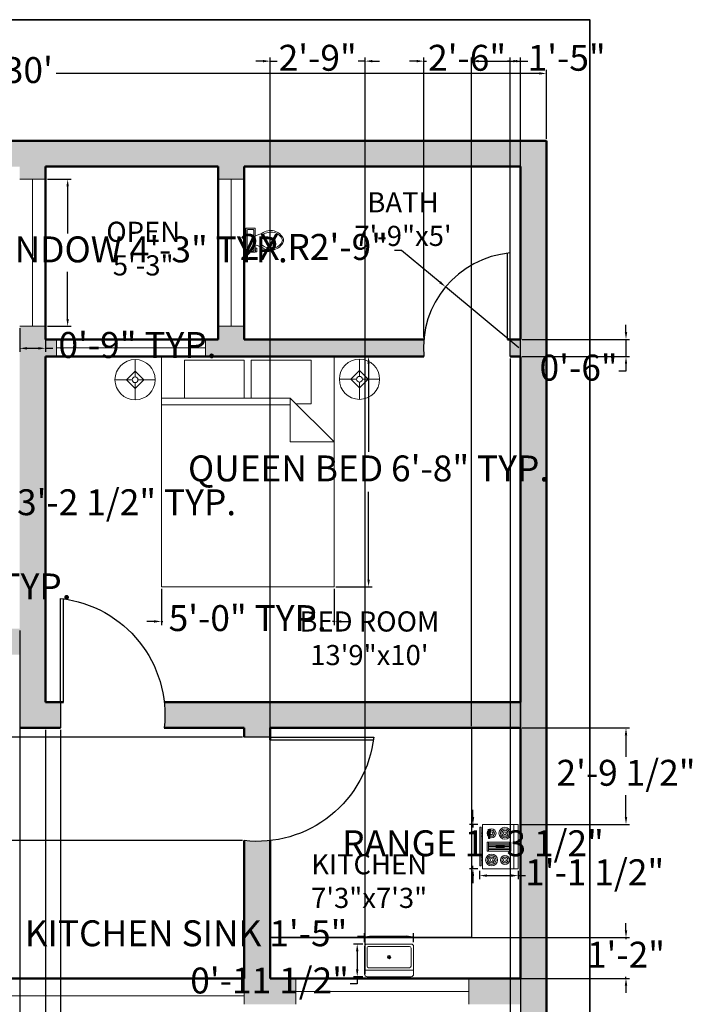
# Model space of a CAD drawing. Units: inches. Extents: x 3695 to 4182, y 4462 to 5050.
# Tile 3 of 3: x 3948 to 4182, y 4708 to 5050. Entities that reach past the tile are written whole.
import ezdxf

# ---------------------------------------------------------------- set-up
doc = ezdxf.new("R2010")
doc.units = ezdxf.units.IN
for name, color, linetype, lineweight in [('A-ANNO-DIMS', 2, 'Continuous', 18), ('A-ANNO-TTLB', 7, 'Continuous', 35), ('A-AREA-IDEN', 7, 'Continuous', 25), ('A-DOOR', 3, 'Continuous', 25), ('A-EQPM', 8, 'Continuous', 18), ('A-FLOR-CASE', 8, 'Continuous', 25), ('A-FLOR-FIXT', 9, 'Continuous', 18), ('A-FURN', 8, 'Continuous', 18), ('A-GLAZ', 4, 'Continuous', 18), ('A-WALL', 7, 'Continuous', 50)]:
    doc.layers.add(name, color=color, linetype=linetype, lineweight=lineweight)
doc.layers.add('A-WALL-PATT', color=18, linetype='Continuous', lineweight=13, true_color=0x000000)
doc.styles.get("Standard").update_dxf_attribs({"font": 'arial.ttf'})
doc.dimstyles.new('ISO-25', dxfattribs={"dimtxt": 9, "dimasz": 2.5, "dimexe": 1.25, "dimexo": 0.625, "dimgap": 2, "dimtad": 0, "dimtih": 1, "dimtoh": 1, "dimdec": 1, "dimlunit": 4, "dimtxsty": 'Standard', "dimcen": 2.5, "dimadec": 0, "dimazin": 0, "dimtfac": 0.5, "dimtdec": 1, "dimtmove": 0, "dimatfit": 3, "dimfxl": 1, "dimarcsym": 0})

# ---------------------------------------------------------------- blocks, each defined once
blk = doc.blocks.new('Bed - Queen')
for p, q in [((0, -80.00003), (0, 0)), ((0, 0), (59.99999, 0)), ((59.99999, 0), (59.99999, -80.00003)), ((7.99999, -1.2), (28.79998, -1.2)), ((7.99999, -14.4), (7.99999, -1.2)), ((28.79998, -1.2), (28.79998, -14.4)), ((31.19999, -1.2), (51.99999, -1.2)), ((31.19999, -14.4), (31.19999, -1.2)), ((51.99999, -1.2), (51.99999, -16.4)), ((0, -14.4), (44.8, -14.4)), ((44.8, -16.8), (0, -16.8)), ((59.99999, -29.6), (44.8, -14.4)), ((44.8, -14.4), (44.8, -29.6)), ((51.99999, -16.4), (46.79936, -16.4)), ((44.8, -29.6), (59.99999, -29.6)), ((59.99999, -80.00003), (0, -80.00003))]:
    blk.add_line(p, q)
blk = doc.blocks.new('Range-Oven - 30 in top')
for p, q in [((0, -3), (30, -3)), ((12, -6), (18, -6)), ((13, -20), (13, -6)), ((14, -6), (14, -20)), ((15, -20), (15, -6)), ((16, -6), (16, -20)), ((17, -20), (17, -6)), ((6, -24), (6, -25)), ((8, -25), (8, -24)), ((18, -20), (12, -20)), ((22, -25), (22, -24)), ((24, -24), (24, -25))]:
    blk.add_line(p, q)
for points in [[(0, -24), (0, 0), (30, 0), (30, -24)], [(12, -21), (12, -5), (18, -5), (18, -21)], [(2, -26), (2, -25), (28, -25), (28, -26)]]:
    blk.add_lwpolyline(points, close=True)
for centre, radius in [((6, -9), 4), ((6, -9), 3), ((24, -9), 3), ((6, -9), 2), ((6, -9), 1), ((24, -9), 2), ((24, -9), 1), ((6, -18), 3), ((6, -18), 2), ((6, -18), 1), ((24, -18), 4), ((24, -18), 3), ((24, -18), 2), ((24, -18), 1)]:
    blk.add_circle(centre, radius)
blk = doc.blocks.new('Sink-single - 30 in top')
blk.add_line((-15, -3.999996), (15, -3.999996))
for points in [[(-13.5, 0), (13.5, 0)], [(-15, -18.499996), (-15, -1.5)], [(-12.5, -5.499996), (12.5, -5.499996)], [(15, -1.5), (15, -18.499996)], [(-13.5, -17.499996), (-13.5, -6.499996)], [(13.5, -6.499996), (13.5, -17.499996)], [(13.5, -19.999996), (-13.5, -19.999996)], [(12.5, -18.499996), (-12.5, -18.499996)]]:
    blk.add_lwpolyline(points)
for radius in [1, 0.5]:
    blk.add_circle((0, -11.999996), radius)
for centre, radius, start, end in [((-13.5, -1.5), 1.5, 90, 180), ((-12.5, -6.499996), 1, 90, 180), ((12.5, -6.499996), 1, 0, 90), ((13.5, -1.5), 1.5, 0, 90), ((-12.5, -17.499996), 1, 180, 270), ((12.5, -17.499996), 1, 270, 0), ((-13.5, -18.499996), 1.5, 180, 270), ((13.5, -18.499996), 1.5, 270, 0)]:
    blk.add_arc(centre, radius, start, end)
blk = doc.blocks.new('*U7')
for p, q in [((-10, -8.5), (-8, -8.5)), ((-10, -9.5), (-10, -8.5)), ((-8, -8.5), (-8, -8)), ((-7, -8), (-7, -9.5)), ((-4, -8), (-6, -14)), ((4, -8), (6, -14)), ((9.5, -6), (9.5, -2)), ((-7, -9.5), (-10, -9.5)), ((4, -14), (-4, -14))]:
    blk.add_line(p, q)
blk.add_lwpolyline([(10.5, -8), (10.5, 0), (-10.5, 0), (-10.5, -8)], close=True)
for points in [[(-9.5, -2), (-9.5, -6)], [(8.5, -1), (-8.5, -1)], [(-8.5, -7), (8.5, -7)]]:
    blk.add_lwpolyline(points)
for centre, radius, start, end in [((-8.62, -1.88), 0.884, 81.8699, 188.1301), ((-8.62, -6.12), 0.884, 171.8699, 278.1301), ((8.62, -1.88), 0.884, 351.8699, 98.1301), ((8.62, -6.12), 0.884, 261.8699, 8.1301), ((3.52, -21.58), 12.17, 141.46911, 247.97143), ((4.2, -21.82), 11.33, 136.36773, 238.94682), ((-3.52, -21.58), 12.17, 292.02843, 38.53071), ((-4.2, -21.82), 11.33, 301.05301, 43.63209), ((0, -27.88), 4, 245.73182, 294.26817), ((0, -29), 4, 254.86053, 285.13947)]:
    blk.add_arc(centre, radius, start, end)
blk = doc.blocks.new('Lamp - Table')
for p, q in [((0, 7), (0, 1)), ((-1, 0), (-7, 0)), ((0, 3), (-3, 0)), ((-3, 0), (0, -3)), ((3, 0), (0, 3)), ((0, -3), (3, 0)), ((1, 0), (7, 0)), ((0, -1), (0, -7))]:
    blk.add_line(p, q)
for radius in [7, 1]:
    blk.add_circle((0, 0), radius)
blk = doc.blocks.new('*D11')
at = {"layer": 'A-ANNO-DIMS', "color": 0, "lineweight": -2, "transparency": 16777216}
for p, q in [((3770.96, 5008.15), (3770.96, 5032.15)), ((4130.96, 5008.15), (4130.96, 5032.15)), ((3773.46, 5030.9), (3941.33, 5030.9)), ((4128.46, 5030.9), (3960.6, 5030.9))]:
    blk.add_line(p, q, dxfattribs=at)
at = {"layer": 'A-ANNO-DIMS', "color": 0, "transparency": 16777216}
for points in [[(3773.46, 5031.31), (3773.46, 5030.48), (3770.96, 5030.9)], [(4128.46, 5031.31), (4128.46, 5030.48), (4130.96, 5030.9)]]:
    blk.add_solid(points, dxfattribs=at)
at = {"layer": 'Defpoints', "color": 0, "transparency": 16777216}
for p in [(4130.96, 5030.9), (3770.96, 5007.52), (4130.96, 5007.52)]:
    blk.add_point(p, dxfattribs=at)
at = {"layer": 'A-ANNO-DIMS', "color": 0, "transparency": 16777216, "insert": (3950.96, 5030.9), "char_height": 9, "attachment_point": 5}
blk.add_mtext("30'", dxfattribs=at)
blk = doc.blocks.new('DOOR-SINGLE-36IN')
for p, q in [((35.25, 9), (35.25, 45)), ((36.25, 9), (36.25, 45)), ((36.25, 9), (36.25, 0))]:
    blk.add_line(p, q)
blk.add_arc((40.75, 4.5), 40.75, 96.3402, 186.3402)
blk = doc.blocks.new('WIN-OPEN-COURT-51IN')
for p, q in [((9, 51.07), (0, 51.07)), ((4.5, 51.07), (4.5, 0)), ((9, 0), (0, 0))]:
    blk.add_line(p, q)
blk = doc.blocks.new('*D17')
at = {"layer": 'A-ANNO-DIMS', "color": 0, "lineweight": -2, "transparency": 16777216}
for p, q in [((3903.58, 4874.02), (3896.2, 4874.02)), ((3897.45, 4871.52), (3897.45, 4858.18)), ((3897.45, 4831.52), (3897.45, 4844.86)), ((3903.58, 4829.02), (3896.2, 4829.02))]:
    blk.add_line(p, q, dxfattribs=at)
at = {"layer": 'A-ANNO-DIMS', "color": 0, "transparency": 16777216}
for points in [[(3897.04, 4871.52), (3897.87, 4871.52), (3897.45, 4874.02)], [(3897.04, 4831.52), (3897.87, 4831.52), (3897.45, 4829.02)]]:
    blk.add_solid(points, dxfattribs=at)
at = {"layer": 'Defpoints', "color": 0, "transparency": 16777216}
for p in [(3897.45, 4874.02), (3904.2, 4874.02), (3904.2, 4829.02)]:
    blk.add_point(p, dxfattribs=at)
at = {"layer": 'A-ANNO-DIMS', "color": 0, "transparency": 16777216, "insert": (3897.45, 4851.52), "char_height": 9, "attachment_point": 5}
blk.add_mtext('SINGLE DOOR 3\'-9" TYP.', dxfattribs=at)
blk = doc.blocks.new('*D18')
at = {"layer": 'A-ANNO-DIMS', "color": 0, "lineweight": -2, "transparency": 16777216}
for p, q in [((3904.2, 4874.65), (3904.2, 4882.02)), ((3942.69, 4874.65), (3942.69, 4882.02)), ((3906.7, 4880.77), (3940.19, 4880.77)), ((3942.69, 4880.77), (3945.19, 4880.77))]:
    blk.add_line(p, q, dxfattribs=at)
at = {"layer": 'A-ANNO-DIMS', "color": 0, "transparency": 16777216}
for points in [[(3906.7, 4881.19), (3906.7, 4880.36), (3904.2, 4880.77)], [(3940.19, 4881.19), (3940.19, 4880.36), (3942.69, 4880.77)]]:
    blk.add_solid(points, dxfattribs=at)
at = {"layer": 'Defpoints', "color": 0, "transparency": 16777216}
for p in [(3942.69, 4880.77), (3904.2, 4874.02), (3942.69, 4874.02)]:
    blk.add_point(p, dxfattribs=at)
at = {"layer": 'A-ANNO-DIMS', "color": 0, "transparency": 16777216, "insert": (3985.1, 4880.77), "char_height": 9, "attachment_point": 5}
blk.add_mtext('3\'-2 1/2" TYP.', dxfattribs=at)
blk = doc.blocks.new('*D21')
at = {"layer": 'A-ANNO-DIMS', "color": 0, "lineweight": -2, "transparency": 16777216}
for p, q in [((4057.81, 4932.52), (4070.43, 4932.52)), ((4069.18, 4930.02), (4069.18, 4899.45)), ((4069.18, 4855.02), (4069.18, 4885.59)), ((4057.81, 4852.52), (4070.43, 4852.52))]:
    blk.add_line(p, q, dxfattribs=at)
at = {"layer": 'A-ANNO-DIMS', "color": 0, "transparency": 16777216}
for points in [[(4068.76, 4930.02), (4069.6, 4930.02), (4069.18, 4932.52)], [(4068.76, 4855.02), (4069.6, 4855.02), (4069.18, 4852.52)]]:
    blk.add_solid(points, dxfattribs=at)
at = {"layer": 'Defpoints', "color": 0, "transparency": 16777216}
for p in [(4057.18, 4932.52), (4069.18, 4932.52), (4057.18, 4852.52)]:
    blk.add_point(p, dxfattribs=at)
at = {"layer": 'A-ANNO-DIMS', "color": 0, "transparency": 16777216, "insert": (4069.18, 4892.52), "char_height": 9, "attachment_point": 5}
blk.add_mtext('QUEEN BED 6\'-8" TYP.', dxfattribs=at)
blk = doc.blocks.new('*D22')
at = {"layer": 'A-ANNO-DIMS', "color": 0, "lineweight": -2, "transparency": 16777216}
for p, q in [((3997.18, 4851.9), (3997.18, 4839.27)), ((4057.18, 4851.9), (4057.18, 4839.27)), ((3994.68, 4840.52), (3992.18, 4840.52)), ((3997.18, 4840.52), (3997.75, 4840.52)), ((4057.18, 4840.52), (4056.61, 4840.52)), ((4059.68, 4840.52), (4062.18, 4840.52))]:
    blk.add_line(p, q, dxfattribs=at)
at = {"layer": 'A-ANNO-DIMS', "color": 0, "transparency": 16777216}
for points in [[(3994.68, 4840.94), (3994.68, 4840.11), (3997.18, 4840.52)], [(4059.68, 4840.94), (4059.68, 4840.11), (4057.18, 4840.52)]]:
    blk.add_solid(points, dxfattribs=at)
at = {"layer": 'Defpoints', "color": 0, "transparency": 16777216}
for p in [(3997.18, 4852.52), (4057.18, 4852.52), (4057.18, 4840.52)]:
    blk.add_point(p, dxfattribs=at)
at = {"layer": 'A-ANNO-DIMS', "color": 0, "transparency": 16777216, "insert": (4027.18, 4840.52), "char_height": 9, "attachment_point": 5}
blk.add_mtext('5\'-0" TYP.', dxfattribs=at)
blk = doc.blocks.new('*D23')
at = {"layer": 'A-ANNO-DIMS', "color": 0, "lineweight": -2, "transparency": 16777216}
for p, q in [((3957.59, 4994.14), (3965.88, 4994.14)), ((3964.63, 4991.64), (3964.63, 4975.27)), ((3964.63, 4945.57), (3964.63, 4961.95)), ((3957.59, 4943.07), (3965.88, 4943.07))]:
    blk.add_line(p, q, dxfattribs=at)
at = {"layer": 'A-ANNO-DIMS', "color": 0, "transparency": 16777216}
for points in [[(3964.21, 4991.64), (3965.04, 4991.64), (3964.63, 4994.14)], [(3964.21, 4945.57), (3965.04, 4945.57), (3964.63, 4943.07)]]:
    blk.add_solid(points, dxfattribs=at)
at = {"layer": 'Defpoints', "color": 0, "transparency": 16777216}
for p in [(3956.96, 4994.14), (3964.63, 4994.14), (3956.96, 4943.07)]:
    blk.add_point(p, dxfattribs=at)
at = {"layer": 'A-ANNO-DIMS', "color": 0, "transparency": 16777216, "insert": (3964.63, 4968.61), "char_height": 9, "attachment_point": 5}
blk.add_mtext('COURT WINDOW 4\'-3" TYP.', dxfattribs=at)
blk = doc.blocks.new('*D24')
at = {"layer": 'A-ANNO-DIMS', "color": 0, "lineweight": -2, "transparency": 16777216}
for p, q in [((3947.96, 4942.44), (3947.96, 4934.16)), ((3956.96, 4942.44), (3956.96, 4934.16)), ((3950.46, 4935.41), (3954.46, 4935.41)), ((3956.96, 4935.41), (3959.46, 4935.41))]:
    blk.add_line(p, q, dxfattribs=at)
at = {"layer": 'A-ANNO-DIMS', "color": 0, "transparency": 16777216}
for points in [[(3950.46, 4935.83), (3950.46, 4934.99), (3947.96, 4935.41)], [(3954.46, 4935.83), (3954.46, 4934.99), (3956.96, 4935.41)]]:
    blk.add_solid(points, dxfattribs=at)
at = {"layer": 'Defpoints', "color": 0, "transparency": 16777216}
for p in [(3947.96, 4943.07), (3956.96, 4943.07), (3956.96, 4935.41)]:
    blk.add_point(p, dxfattribs=at)
at = {"layer": 'A-ANNO-DIMS', "color": 0, "transparency": 16777216, "insert": (3988.89, 4935.41), "char_height": 9, "attachment_point": 5}
blk.add_mtext('0\'-9" TYP.', dxfattribs=at)
blk = doc.blocks.new('*D25')
at = {"layer": 'A-ANNO-DIMS', "color": 0, "lineweight": -2, "transparency": 16777216}
for p, q in [((4105.45, 4772.54), (4105.45, 4775.04)), ((4107.15, 4770.04), (4104.2, 4770.04)), ((4105.45, 4770.04), (4105.45, 4768.95)), ((4107.15, 4754.55), (4104.2, 4754.55)), ((4105.45, 4754.55), (4105.45, 4755.64)), ((4105.45, 4752.05), (4105.45, 4749.55))]:
    blk.add_line(p, q, dxfattribs=at)
at = {"layer": 'A-ANNO-DIMS', "color": 0, "transparency": 16777216}
for points in [[(4105.03, 4772.54), (4105.87, 4772.54), (4105.45, 4770.04)], [(4105.03, 4752.05), (4105.87, 4752.05), (4105.45, 4754.55)]]:
    blk.add_solid(points, dxfattribs=at)
at = {"layer": 'Defpoints', "color": 0, "transparency": 16777216}
for p in [(4107.77, 4770.04), (4105.45, 4754.55), (4107.77, 4754.55)]:
    blk.add_point(p, dxfattribs=at)
at = {"layer": 'A-ANNO-DIMS', "color": 0, "transparency": 16777216, "insert": (4105.45, 4762.3), "char_height": 9, "attachment_point": 5}
blk.add_mtext('RANGE 1\'-3 1/2"', dxfattribs=at)
blk = doc.blocks.new('*D26')
at = {"layer": 'A-ANNO-DIMS', "color": 0, "lineweight": -2, "transparency": 16777216}
for p, q in [((4107.77, 4753.93), (4107.77, 4750.98)), ((4110.27, 4752.23), (4118.7, 4752.23)), ((4121.2, 4753.93), (4121.2, 4750.98)), ((4121.2, 4752.23), (4123.7, 4752.23))]:
    blk.add_line(p, q, dxfattribs=at)
at = {"layer": 'A-ANNO-DIMS', "color": 0, "transparency": 16777216}
for points in [[(4110.27, 4752.65), (4110.27, 4751.81), (4107.77, 4752.23)], [(4118.7, 4752.65), (4118.7, 4751.81), (4121.2, 4752.23)]]:
    blk.add_solid(points, dxfattribs=at)
at = {"layer": 'Defpoints', "color": 0, "transparency": 16777216}
for p in [(4107.77, 4754.55), (4121.2, 4754.55), (4121.2, 4752.23)]:
    blk.add_point(p, dxfattribs=at)
at = {"layer": 'A-ANNO-DIMS', "color": 0, "transparency": 16777216, "insert": (4147.72, 4752.23), "char_height": 9, "attachment_point": 5}
blk.add_mtext('1\'-1 1/2"', dxfattribs=at)
blk = doc.blocks.new('*D27')
at = {"layer": 'A-ANNO-DIMS', "color": 0, "lineweight": -2, "transparency": 16777216}
for p, q in [((4067.78, 4731.03), (4065.28, 4731.03)), ((4067.78, 4729.1), (4067.78, 4732.28)), ((4082.31, 4731.03), (4070.28, 4731.03)), ((4084.81, 4729.1), (4084.81, 4732.28))]:
    blk.add_line(p, q, dxfattribs=at)
at = {"layer": 'A-ANNO-DIMS', "color": 0, "transparency": 16777216}
for points in [[(4070.28, 4731.44), (4070.28, 4730.61), (4067.78, 4731.03)], [(4082.31, 4731.44), (4082.31, 4730.61), (4084.81, 4731.03)]]:
    blk.add_solid(points, dxfattribs=at)
at = {"layer": 'Defpoints', "color": 0, "transparency": 16777216}
for p in [(4067.78, 4731.03), (4067.78, 4728.47), (4084.81, 4728.47)]:
    blk.add_point(p, dxfattribs=at)
at = {"layer": 'A-ANNO-DIMS', "color": 0, "transparency": 16777216, "insert": (4005.76, 4731.03), "char_height": 9, "attachment_point": 5}
blk.add_mtext('KITCHEN SINK 1\'-5"', dxfattribs=at)
blk = doc.blocks.new('*D28')
at = {"layer": 'A-ANNO-DIMS', "color": 0, "lineweight": -2, "transparency": 16777216}
for p, q in [((4067.16, 4728.47), (4063.98, 4728.47)), ((4065.23, 4725.97), (4065.23, 4719.62)), ((4067.16, 4717.12), (4063.98, 4717.12)), ((4065.23, 4717.12), (4065.23, 4714.62)), ((4065.23, 4714.62), (4062.73, 4714.62))]:
    blk.add_line(p, q, dxfattribs=at)
at = {"layer": 'A-ANNO-DIMS', "color": 0, "transparency": 16777216}
for points in [[(4064.81, 4725.97), (4065.65, 4725.97), (4065.23, 4728.47)], [(4064.81, 4719.62), (4065.65, 4719.62), (4065.23, 4717.12)]]:
    blk.add_solid(points, dxfattribs=at)
at = {"layer": 'Defpoints', "color": 0, "transparency": 16777216}
for p in [(4067.78, 4728.47), (4065.23, 4717.12), (4067.78, 4717.12)]:
    blk.add_point(p, dxfattribs=at)
at = {"layer": 'A-ANNO-DIMS', "color": 0, "transparency": 16777216, "insert": (4034.79, 4714.62), "char_height": 9, "attachment_point": 5}
blk.add_mtext('0\'-11 1/2"', dxfattribs=at)
blk = doc.blocks.new('*D40')
at = {"layer": 'A-ANNO-DIMS', "color": 0, "lineweight": -2, "transparency": 16777216}
for p, q in [((4025.34, 4800.38), (3742.06, 4800.38)), ((3743.31, 4797.88), (3743.31, 4788.98)), ((3743.31, 4766.88), (3743.31, 4775.78)), ((4025.34, 4764.38), (3742.06, 4764.38))]:
    blk.add_line(p, q, dxfattribs=at)
at = {"layer": 'A-ANNO-DIMS', "color": 0, "transparency": 16777216}
for points in [[(3742.9, 4797.88), (3743.73, 4797.88), (3743.31, 4800.38)], [(3742.9, 4766.88), (3743.73, 4766.88), (3743.31, 4764.38)]]:
    blk.add_solid(points, dxfattribs=at)
at = {"layer": 'Defpoints', "color": 0, "transparency": 16777216}
for p in [(3743.31, 4800.38), (4025.96, 4800.38), (4025.96, 4764.38)]:
    blk.add_point(p, dxfattribs=at)
at = {"layer": 'A-ANNO-DIMS', "color": 0, "transparency": 16777216, "insert": (3743.31, 4782.38), "char_height": 9, "attachment_point": 5}
blk.add_mtext('3\'-0"', dxfattribs=at)
blk = doc.blocks.new('*D41')
at = {"layer": 'A-ANNO-DIMS', "color": 0, "lineweight": -2, "transparency": 16777216}
for p, q in [((3956.96, 4802.9), (3956.96, 4474.62)), ((3962.16, 4802.9), (3962.16, 4474.62)), ((3954.46, 4475.87), (3951.96, 4475.87)), ((3956.96, 4475.87), (3962.16, 4475.87)), ((3964.66, 4475.87), (3967.16, 4475.87))]:
    blk.add_line(p, q, dxfattribs=at)
at = {"layer": 'A-ANNO-DIMS', "color": 0, "transparency": 16777216}
for points in [[(3954.46, 4476.29), (3954.46, 4475.46), (3956.96, 4475.87)], [(3964.66, 4476.29), (3964.66, 4475.46), (3962.16, 4475.87)]]:
    blk.add_solid(points, dxfattribs=at)
at = {"layer": 'Defpoints', "color": 0, "transparency": 16777216}
for p in [(3956.96, 4803.52), (3962.16, 4803.52), (3962.16, 4475.87)]:
    blk.add_point(p, dxfattribs=at)
at = {"layer": 'A-ANNO-DIMS', "color": 0, "transparency": 16777216, "insert": (3981.12, 4475.87), "char_height": 9, "attachment_point": 5}
blk.add_mtext('0\'-5"', dxfattribs=at)
blk = doc.blocks.new('*D42')
at = {"layer": 'A-ANNO-DIMS', "color": 0, "lineweight": -2, "transparency": 16777216}
for p, q in [((3942.69, 4837.4), (3942.69, 4474.62)), ((3947.96, 4837.4), (3947.96, 4474.62)), ((3940.19, 4475.87), (3937.69, 4475.87)), ((3942.69, 4475.87), (3947.96, 4475.87)), ((3950.46, 4475.87), (3952.96, 4475.87))]:
    blk.add_line(p, q, dxfattribs=at)
at = {"layer": 'A-ANNO-DIMS', "color": 0, "transparency": 16777216}
for points in [[(3940.19, 4476.29), (3940.19, 4475.46), (3942.69, 4475.87)], [(3950.46, 4476.29), (3950.46, 4475.46), (3947.96, 4475.87)]]:
    blk.add_solid(points, dxfattribs=at)
at = {"layer": 'Defpoints', "color": 0, "transparency": 16777216}
for p in [(3942.69, 4838.02), (3947.96, 4838.02), (3947.96, 4475.87)]:
    blk.add_point(p, dxfattribs=at)
at = {"layer": 'A-ANNO-DIMS', "color": 0, "transparency": 16777216, "insert": (3977.41, 4475.87), "char_height": 9, "attachment_point": 5}
blk.add_mtext('0\'-5 1/2"', dxfattribs=at)
blk = doc.blocks.new('*D43')
at = {"layer": 'A-ANNO-DIMS', "color": 0, "lineweight": -2, "transparency": 16777216}
for p, q in [((4158.61, 4941.02), (4158.61, 4943.52)), ((4122.59, 4938.52), (4159.86, 4938.52)), ((4158.61, 4938.52), (4158.61, 4932.52)), ((4122.59, 4932.52), (4159.86, 4932.52)), ((4158.61, 4930.02), (4158.61, 4927.52)), ((4158.61, 4927.52), (4156.11, 4927.52))]:
    blk.add_line(p, q, dxfattribs=at)
at = {"layer": 'A-ANNO-DIMS', "color": 0, "transparency": 16777216}
for points in [[(4158.2, 4941.02), (4159.03, 4941.02), (4158.61, 4938.52)], [(4158.2, 4930.02), (4159.03, 4930.02), (4158.61, 4932.52)]]:
    blk.add_solid(points, dxfattribs=at)
at = {"layer": 'Defpoints', "color": 0, "transparency": 16777216}
for p in [(4121.96, 4938.52), (4121.96, 4932.52), (4158.61, 4932.52)]:
    blk.add_point(p, dxfattribs=at)
at = {"layer": 'A-ANNO-DIMS', "color": 0, "transparency": 16777216, "insert": (4142.15, 4927.52), "char_height": 9, "attachment_point": 5}
blk.add_mtext('0\'-6"', dxfattribs=at)
blk = doc.blocks.new('*D44')
at = {"layer": 'A-ANNO-DIMS', "color": 0, "lineweight": -2, "transparency": 16777216}
for p, q in [((4085.9, 5035.17), (4083.4, 5035.17)), ((4088.4, 4939.15), (4088.4, 5036.42)), ((4088.4, 5035.17), (4089.36, 5035.17)), ((4118.4, 5035.17), (4117.44, 5035.17)), ((4118.4, 4939.15), (4118.4, 5036.42)), ((4120.9, 5035.17), (4123.4, 5035.17))]:
    blk.add_line(p, q, dxfattribs=at)
at = {"layer": 'A-ANNO-DIMS', "color": 0, "transparency": 16777216}
for points in [[(4085.9, 5035.59), (4085.9, 5034.76), (4088.4, 5035.17)], [(4120.9, 5035.59), (4120.9, 5034.76), (4118.4, 5035.17)]]:
    blk.add_solid(points, dxfattribs=at)
at = {"layer": 'Defpoints', "color": 0, "transparency": 16777216}
for p in [(4118.4, 5035.17), (4088.4, 4938.52), (4118.4, 4938.52)]:
    blk.add_point(p, dxfattribs=at)
at = {"layer": 'A-ANNO-DIMS', "color": 0, "transparency": 16777216, "insert": (4103.4, 5035.17), "char_height": 9, "attachment_point": 5}
blk.add_mtext('2\'-6"', dxfattribs=at)
blk = doc.blocks.new('*D46')
at = {"layer": 'A-ANNO-DIMS', "color": 0, "lineweight": -2, "transparency": 16777216}
for p, q in [((4104.89, 4804.15), (4104.89, 5036.42)), ((4107.39, 5035.17), (4119.46, 5035.17)), ((4121.96, 4804.15), (4121.96, 5036.42)), ((4121.96, 5035.17), (4124.46, 5035.17))]:
    blk.add_line(p, q, dxfattribs=at)
at = {"layer": 'A-ANNO-DIMS', "color": 0, "transparency": 16777216}
for points in [[(4107.39, 5035.59), (4107.39, 5034.76), (4104.89, 5035.17)], [(4119.46, 5035.59), (4119.46, 5034.76), (4121.96, 5035.17)]]:
    blk.add_solid(points, dxfattribs=at)
at = {"layer": 'Defpoints', "color": 0, "transparency": 16777216}
for p in [(4121.96, 5035.17), (4104.89, 4803.52), (4121.96, 4803.52)]:
    blk.add_point(p, dxfattribs=at)
at = {"layer": 'A-ANNO-DIMS', "color": 0, "transparency": 16777216, "insert": (4138, 5035.17), "char_height": 9, "attachment_point": 5}
blk.add_mtext('1\'-5"', dxfattribs=at)
blk = doc.blocks.new('*D47')
at = {"layer": 'A-ANNO-DIMS', "color": 0, "lineweight": -2, "transparency": 16777216}
for p, q in [((4158.61, 4733.18), (4158.61, 4735.68)), ((4035.59, 4730.68), (4159.86, 4730.68)), ((4158.61, 4730.68), (4158.61, 4730.12)), ((4158.61, 4716.52), (4158.61, 4717.08)), ((4035.59, 4716.52), (4159.86, 4716.52)), ((4158.61, 4714.02), (4158.61, 4711.52))]:
    blk.add_line(p, q, dxfattribs=at)
at = {"layer": 'A-ANNO-DIMS', "color": 0, "transparency": 16777216}
for points in [[(4158.2, 4733.18), (4159.03, 4733.18), (4158.61, 4730.68)], [(4158.2, 4714.02), (4159.03, 4714.02), (4158.61, 4716.52)]]:
    blk.add_solid(points, dxfattribs=at)
at = {"layer": 'Defpoints', "color": 0, "transparency": 16777216}
for p in [(4034.96, 4730.68), (4158.61, 4730.68), (4034.96, 4716.52)]:
    blk.add_point(p, dxfattribs=at)
at = {"layer": 'A-ANNO-DIMS', "color": 0, "transparency": 16777216, "insert": (4158.61, 4723.6), "char_height": 9, "attachment_point": 5}
blk.add_mtext('1\'-2"', dxfattribs=at)
blk = doc.blocks.new('*D48')
at = {"layer": 'A-ANNO-DIMS', "color": 0, "lineweight": -2, "transparency": 16777216}
for p, q in [((4122.59, 4803.52), (4159.86, 4803.52)), ((4158.61, 4801.02), (4158.61, 4793.44)), ((4158.61, 4772.54), (4158.61, 4780.13)), ((4121.82, 4770.04), (4159.86, 4770.04))]:
    blk.add_line(p, q, dxfattribs=at)
at = {"layer": 'A-ANNO-DIMS', "color": 0, "transparency": 16777216}
for points in [[(4158.2, 4801.02), (4159.03, 4801.02), (4158.61, 4803.52)], [(4158.2, 4772.54), (4159.03, 4772.54), (4158.61, 4770.04)]]:
    blk.add_solid(points, dxfattribs=at)
at = {"layer": 'Defpoints', "color": 0, "transparency": 16777216}
for p in [(4121.96, 4803.52), (4158.61, 4803.52), (4121.2, 4770.04)]:
    blk.add_point(p, dxfattribs=at)
at = {"layer": 'A-ANNO-DIMS', "color": 0, "transparency": 16777216, "insert": (4158.61, 4786.78), "char_height": 9, "attachment_point": 5}
blk.add_mtext('2\'-9 1/2"', dxfattribs=at)
blk = doc.blocks.new('*D49')
at = {"layer": 'A-ANNO-DIMS', "color": 0, "lineweight": -2, "transparency": 16777216}
for p, q in [((4032.46, 5035.17), (4029.96, 5035.17)), ((4034.96, 4717.15), (4034.96, 5036.42)), ((4034.96, 5035.17), (4037.46, 5035.17)), ((4068.03, 5035.17), (4065.54, 5035.17)), ((4068.03, 4717.99), (4068.03, 5036.42)), ((4070.53, 5035.17), (4073.03, 5035.17))]:
    blk.add_line(p, q, dxfattribs=at)
at = {"layer": 'A-ANNO-DIMS', "color": 0, "transparency": 16777216}
for points in [[(4032.46, 5035.59), (4032.46, 5034.76), (4034.96, 5035.17)], [(4070.53, 5035.59), (4070.53, 5034.76), (4068.03, 5035.17)]]:
    blk.add_solid(points, dxfattribs=at)
at = {"layer": 'Defpoints', "color": 0, "transparency": 16777216}
for p in [(4068.03, 5035.17), (4068.03, 4717.37), (4034.96, 4716.52)]:
    blk.add_point(p, dxfattribs=at)
at = {"layer": 'A-ANNO-DIMS', "color": 0, "transparency": 16777216, "insert": (4051.5, 5035.17), "char_height": 9, "attachment_point": 5}
blk.add_mtext('2\'-9"', dxfattribs=at)
blk = doc.blocks.new('*D50')
at = {"layer": 'A-ANNO-DIMS', "color": 0, "lineweight": -2, "transparency": 16777216}
for p, q in [((4118.4, 4931.9), (4118.4, 4474.62)), ((4121.96, 4931.9), (4121.96, 4474.62)), ((4115.9, 4475.87), (4113.4, 4475.87)), ((4118.4, 4475.87), (4121.96, 4475.87)), ((4124.46, 4475.87), (4126.96, 4475.87))]:
    blk.add_line(p, q, dxfattribs=at)
at = {"layer": 'A-ANNO-DIMS', "color": 0, "transparency": 16777216}
for points in [[(4115.9, 4476.29), (4115.9, 4475.46), (4118.4, 4475.87)], [(4124.46, 4476.29), (4124.46, 4475.46), (4121.96, 4475.87)]]:
    blk.add_solid(points, dxfattribs=at)
at = {"layer": 'Defpoints', "color": 0, "transparency": 16777216}
for p in [(4118.4, 4932.52), (4121.96, 4932.52), (4121.96, 4475.87)]:
    blk.add_point(p, dxfattribs=at)
at = {"layer": 'A-ANNO-DIMS', "color": 0, "transparency": 16777216, "insert": (4151.41, 4475.87), "char_height": 9, "attachment_point": 5}
blk.add_mtext('0\'-3 1/2"', dxfattribs=at)
blk = doc.blocks.new('*D55')
at = {"layer": 'A-ANNO-DIMS', "color": 0, "lineweight": -2, "transparency": 16777216}
for p, q in [((4078.17, 4969.46), (4080.67, 4969.46)), ((4080.67, 4969.46), (4094.02, 4958.34)), ((4121.4, 4935.52), (4095.94, 4956.74))]:
    blk.add_line(p, q, dxfattribs=at)
at = {"layer": 'A-ANNO-DIMS', "color": 0, "transparency": 16777216}
blk.add_solid([(4094.29, 4958.66), (4093.75, 4958.02), (4095.94, 4956.74)], dxfattribs=at)
at = {"layer": 'Defpoints', "color": 0, "transparency": 16777216}
for p in [(4095.94, 4956.74), (4121.4, 4935.52)]:
    blk.add_point(p, dxfattribs=at)
at = {"layer": 'A-ANNO-DIMS', "color": 0, "transparency": 16777216, "insert": (4050.15, 4969.46), "char_height": 9, "attachment_point": 5}
blk.add_mtext('2X R2\'-9"', dxfattribs=at)

msp = doc.modelspace()

# ---------------------------------------------------------------- hatches: boundary and pattern name
at = {"layer": 'A-WALL-PATT'}
h = msp.add_hatch(color=256, dxfattribs=at)
h.dxf.hatch_style = 1
h.paths.add_polyline_path([(3906.69, 4838.02), (3779.96, 4838.02), (3779.96, 4998.52), (3947.96, 4998.52), (3947.96, 4994.14), (3956.96, 4994.14), (3956.96, 4998.52), (4016.96, 4998.52), (4016.96, 4994.14), (4025.96, 4994.14), (4025.96, 4998.52), (4121.96, 4998.52), (4121.96, 4938.52), (4118.4, 4938.52), (4118.4, 4932.52), (4121.96, 4932.52), (4121.96, 4812.52), (4025.96, 4812.52), (3998.16, 4812.52, -0.055385), (3998.16, 4803.52), (4025.96, 4803.52), (4025.96, 4800.38), (4034.96, 4800.38), (4034.96, 4803.52), (4121.96, 4803.52), (4121.96, 4716.52), (4103.96, 4716.52), (4103.96, 4707.52), (4121.96, 4707.52), (4121.96, 4512.52), (4111.49, 4512.52), (4111.49, 4503.52), (4130.96, 4503.52), (4130.96, 5007.52), (3770.96, 5007.52), (3770.96, 4503.52), (4004.7, 4503.52), (4004.7, 4512.52), (3860.96, 4512.52), (3860.96, 4529.52), (3851.96, 4529.52), (3851.96, 4512.52), (3779.96, 4512.52), (3779.96, 4570.52), (3784.38, 4570.52), (3784.38, 4579.52), (3779.96, 4579.52), (3779.96, 4707.52), (3908.96, 4707.52), (3908.96, 4716.52), (3779.96, 4716.52), (3779.96, 4829.02), (3906.69, 4829.02, -0.055385)])
h.paths.add_polyline_path([(4034.96, 4764.38, -0.055385), (4025.96, 4764.38), (4025.96, 4716.52), (4025.96, 4707.52), (4043.96, 4707.52), (4043.96, 4716.52), (4034.96, 4716.52)], flags=17)
h = msp.add_hatch(color=256, dxfattribs=at)
h.dxf.hatch_style = 1
h.paths.add_polyline_path([(3956.96, 4932.52), (3960.75, 4932.52), (3960.75, 4938.52), (3956.96, 4938.52), (3956.96, 4943.07), (3947.96, 4943.07), (3947.96, 4838.02), (3942.69, 4838.02), (3942.69, 4829.02), (3947.96, 4829.02), (3947.96, 4803.52), (3956.96, 4803.52), (3962.16, 4803.52), (3962.16, 4812.52), (3956.96, 4812.52), (3956.96, 4829.02)])
h.paths.add_polyline_path([(4088.4, 4938.52), (4025.96, 4938.52), (4025.96, 4943.07), (4016.96, 4943.07), (4016.96, 4938.52), (4012.55, 4938.52), (4012.55, 4932.52), (4057.18, 4932.52), (4088.4, 4932.52, -0.045361)])

# ---------------------------------------------------------------- linework, layer by layer
at = {"layer": 'A-ANNO-TTLB'}
msp.add_lwpolyline([(3718.2, 5049.57), (4146.02, 5049.57), (4146.02, 4481.47), (3718.2, 4481.47)], close=True, dxfattribs=at)
at = {"layer": 'A-DOOR'}
for p, q in [((4117.4, 4938.52), (4117.4, 4968.52)), ((4118.4, 4938.52), (4118.4, 4968.52)), ((4118.4, 4932.52), (4118.4, 4938.52))]:
    msp.add_line(p, q, dxfattribs=at)
msp.add_arc((4121.4, 4935.52), 33.14, 95.1944, 185.1944, dxfattribs=at)
at = {"layer": 'A-FLOR-CASE'}
for p, q in [((4104.89, 4803.52), (4104.89, 4730.68)), ((4104.89, 4730.68), (4034.96, 4730.68))]:
    msp.add_line(p, q, dxfattribs=at)
at = {"layer": 'A-GLAZ'}
for p, q in [((3960.75, 4938.52), (3960.75, 4932.52)), ((4012.55, 4938.52), (4012.55, 4932.52)), ((3960.75, 4935.52), (4012.55, 4935.52)), ((4025.96, 4716.52), (4025.96, 4707.52)), ((4043.96, 4707.52), (4043.96, 4716.52)), ((4043.96, 4716.52), (4043.96, 4707.52)), ((4103.96, 4707.52), (4103.96, 4716.52)), ((4025.96, 4710.52), (3908.96, 4710.52)), ((4043.96, 4712.02), (4103.96, 4712.02))]:
    msp.add_line(p, q, dxfattribs=at)
at = {"layer": 'A-WALL'}
for p, q in [((3770.96, 5007.52), (4130.96, 5007.52)), ((4130.96, 5007.52), (4130.96, 4503.52)), ((3956.96, 4998.52), (4016.96, 4998.52)), ((3956.96, 4938.52), (3956.96, 4998.52)), ((4016.96, 4938.52), (4016.96, 4998.52)), ((4025.96, 4998.52), (4121.96, 4998.52)), ((4025.96, 4938.52), (4025.96, 4998.52)), ((4121.96, 4998.52), (4121.96, 4938.52)), ((3956.96, 4938.52), (4016.96, 4938.52)), ((4025.96, 4938.52), (4088.4, 4938.52)), ((4117.4, 4938.52), (4121.96, 4938.52)), ((3956.96, 4829.02), (3956.96, 4932.52)), ((3956.96, 4932.52), (4016.96, 4932.52)), ((4016.96, 4932.52), (4025.96, 4932.52)), ((4025.96, 4932.52), (4088.4, 4932.52)), ((4118.4, 4932.52), (4121.96, 4932.52)), ((4121.96, 4932.52), (4121.96, 4812.52)), ((3956.96, 4829.02), (3956.96, 4812.52)), ((3956.96, 4812.52), (3963.16, 4812.52)), ((3998.16, 4812.52), (4121.96, 4812.52)), ((4025.96, 4812.52), (4121.96, 4812.52)), ((3956.96, 4803.52), (3947.96, 4803.52)), ((3956.96, 4803.52), (3962.16, 4803.52)), ((3998.16, 4803.52), (4025.96, 4803.52)), ((4025.96, 4803.52), (4025.96, 4800.38)), ((4034.96, 4803.52), (4034.96, 4799.38)), ((4034.96, 4803.52), (4121.96, 4803.52)), ((4121.96, 4803.52), (4121.96, 4716.52)), ((4025.96, 4764.38), (4025.96, 4716.52)), ((4034.96, 4764.38), (4034.96, 4716.52)), ((4025.96, 4716.52), (3779.96, 4716.52)), ((4034.96, 4716.52), (4121.96, 4716.52))]:
    msp.add_line(p, q, dxfattribs=at)

# ---------------------------------------------------------------- block references
at = {"layer": 'A-DOOR', "extrusion": (0, 0, -1), "zscale": -1}
msp.add_blockref('DOOR-SINGLE-36IN', (-3998.41, 4803.52), dxfattribs=at)
at = {"layer": 'A-DOOR', "extrusion": (0, 0, -1), "zscale": -1, "rotation": 90.00000000000227}
msp.add_blockref('DOOR-SINGLE-36IN', (-4025.96, 4764.13), dxfattribs=at)
at = {"layer": 'A-EQPM', "xscale": 0.5163314572999419, "yscale": 0.5163314572999419, "zscale": 0.5163314572999419, "rotation": 270}
msp.add_blockref('Range-Oven - 30 in top', (4121.2, 4770.04), dxfattribs=at)
at = {"layer": 'A-FLOR-FIXT'}
for name, p, xscale, yscale, zscale, rotation in [('*U7', (4026.55, 4972.93), 0.3973700613755364, 0.3973700613755364, 0.3973700613755364, 90), ('Sink-single - 30 in top', (4076.3, 4717.12), 0.5676401924244903, 0.5676401924244903, 0.5676401924244903, 180)]:
    msp.add_blockref(name, p, dxfattribs=dict(at, xscale=xscale, yscale=yscale, zscale=zscale, rotation=rotation))
at = {"layer": 'A-FURN'}
for name, p in [('Bed - Queen', (3997.18, 4932.52)), ('Lamp - Table', (3988.06, 4924.5)), ('Lamp - Table', (4066.02, 4924.66))]:
    msp.add_blockref(name, p, dxfattribs=at)
at = {"layer": 'A-GLAZ'}
msp.add_blockref('WIN-OPEN-COURT-51IN', (3947.96, 4943.07), dxfattribs=at)
at = {"layer": 'A-GLAZ', "rotation": 180}
msp.add_blockref('WIN-OPEN-COURT-51IN', (4025.96, 4994.14), dxfattribs=at)

# ---------------------------------------------------------------- texts
at = {"layer": 'A-AREA-IDEN', "char_height": 7, "attachment_point": 1}
for s, width, insert in [('\\pxqc;{\\fArial|b1|i0|c0|p34;BATH\\P7\'-9"x5\'}', 72.5405, (4044.86, 4989.63)), ('\\pxqc;{\\fArial|b1|i0|c0|p34;OPEN\\P5\'-3"}', 52.1782, (3964.79, 4979.39)), ('\\pxqc;{\\fArial|b1|i0|c0|p34;BED ROOM\\P13\'9"x10\'}', 82.7777, (4028.06, 4844.02)), ('\\pxqc;{\\fArial|b1|i0|c0|p34;KITCHEN\\P7\'3"x7\'3"}', 60.5751, (4039.09, 4759.66))]:
    msp.add_mtext_dynamic_manual_height_columns(s, width=width, gutter_width=12.5, heights=[0], dxfattribs=dict(at, insert=insert))

# ---------------------------------------------------------------- dimensions: what is measured, and where the dimension line sits
at = {"layer": 'A-ANNO-DIMS'}
for base, p1, p2, override, picture, middle in [((4068.03, 5035.17), (4034.96, 4716.52), (4068.03, 4717.37), {"dimdec": 1, "dimlfac": 1, "dimrnd": 0, "dimzin": 1, "dimdsep": 46, "dimlunit": 4, "dimfrac": 2}, '*D49', (4051.5, 5035.17)), ((4118.4, 5035.17), (4088.4, 4938.52), (4118.4, 4938.52), {"dimdec": 1, "dimlfac": 1, "dimrnd": 0, "dimzin": 1, "dimdsep": 46, "dimlunit": 4, "dimfrac": 2}, '*D44', (4103.4, 5035.17)), ((4121.96, 5035.17), (4104.89, 4803.52), (4121.96, 4803.52), {"dimdec": 1, "dimlfac": 1, "dimrnd": 0, "dimzin": 1, "dimdsep": 46, "dimlunit": 4, "dimfrac": 2}, '*D46', (4138, 5035.17)), ((4130.96, 5030.9), (3770.96, 5007.52), (4130.96, 5007.52), {"dimclrd": 0, "dimclre": 0, "dimclrt": 0}, '*D11', (3950.96, 5030.9)), ((4121.96, 4475.87), (4118.4, 4932.52), (4121.96, 4932.52), {"dimdec": 1, "dimlfac": 1, "dimrnd": 0, "dimzin": 1, "dimdsep": 46, "dimlunit": 4, "dimfrac": 2}, '*D50', (4151.41, 4475.87)), ((3947.96, 4475.87), (3942.69, 4838.02), (3947.96, 4838.02), {"dimdec": 1, "dimlfac": 1, "dimrnd": 0, "dimzin": 1, "dimdsep": 46, "dimlunit": 4, "dimfrac": 2}, '*D42', (3977.41, 4475.87)), ((3962.16, 4475.87), (3956.96, 4803.52), (3962.16, 4803.52), {"dimdec": 1, "dimlfac": 1, "dimrnd": 0, "dimzin": 1, "dimdsep": 46, "dimlunit": 4, "dimfrac": 2}, '*D41', (3981.12, 4475.87)), ((4121.2, 4752.23), (4107.77, 4754.55), (4121.2, 4754.55), {"dimdec": 1, "dimlfac": 1, "dimrnd": 0, "dimzin": 1, "dimdsep": 46, "dimlunit": 4, "dimfrac": 2}, '*D26', (4147.72, 4752.23))]:
    dim = msp.add_linear_dim(base=base, p1=p1, p2=p2, dimstyle='ISO-25', override=override, dxfattribs=at)
    dim.commit()
    dim.dimension.update_dxf_attribs({"geometry": picture, "text_midpoint": middle})
for base, p1, p2, angle, text, picture, middle in [((3964.63, 4994.14), (3956.96, 4943.07), (3956.96, 4994.14), 90, 'COURT WINDOW <> TYP.', '*D23', (3964.63, 4968.61)), ((4069.18, 4932.52), (4057.18, 4852.52), (4057.18, 4932.52), 90, 'QUEEN BED <> TYP.', '*D21', (4069.18, 4892.52)), ((3897.45, 4874.02), (3904.2, 4829.02), (3904.2, 4874.02), 90, 'SINGLE DOOR <> TYP.', '*D17', (3897.45, 4851.52)), ((4105.45, 4754.55), (4107.77, 4770.04), (4107.77, 4754.55), 270, 'RANGE <>', '*D25', (4105.45, 4762.3)), ((4067.78, 4731.03), (4084.81, 4728.47), (4067.78, 4728.47), 180, 'KITCHEN SINK <>', '*D27', (4005.76, 4731.03))]:
    dim = msp.add_linear_dim(base=base, p1=p1, p2=p2, angle=angle, text=text, dimstyle='ISO-25', override={"dimdec": 1, "dimlfac": 1, "dimrnd": 0, "dimzin": 1, "dimdsep": 46, "dimlunit": 4, "dimfrac": 2}, dxfattribs=at)
    dim.commit()
    dim.dimension.update_dxf_attribs({"geometry": picture, "text_midpoint": middle})
dim = msp.add_radius_dim(center=(4121.4, 4935.52), mpoint=(4095.94, 4956.74), text='2X <>', dimstyle='ISO-25', override={"dimdec": 1, "dimlfac": 1, "dimrnd": 0, "dimzin": 1, "dimdsep": 46, "dimlunit": 4, "dimfrac": 2}, dxfattribs=at)
dim.commit()
dim.dimension.update_dxf_attribs({"geometry": '*D55', "text_midpoint": (4050.15, 4969.46), "dimtype": 164})
for base, p1, p2, picture, middle in [((3956.96, 4935.41), (3947.96, 4943.07), (3956.96, 4943.07), '*D24', (3988.89, 4935.41)), ((3942.69, 4880.77), (3904.2, 4874.02), (3942.69, 4874.02), '*D18', (3985.1, 4880.77)), ((4057.18, 4840.52), (3997.18, 4852.52), (4057.18, 4852.52), '*D22', (4027.18, 4840.52))]:
    dim = msp.add_linear_dim(base=base, p1=p1, p2=p2, text='<> TYP.', dimstyle='ISO-25', override={"dimdec": 1, "dimlfac": 1, "dimrnd": 0, "dimzin": 1, "dimdsep": 46, "dimlunit": 4, "dimfrac": 2}, dxfattribs=at)
    dim.commit()
    dim.dimension.update_dxf_attribs({"geometry": picture, "text_midpoint": middle})
for base, p1, p2, angle, picture, middle in [((4158.61, 4932.52), (4121.96, 4938.52), (4121.96, 4932.52), 90, '*D43', (4142.15, 4927.52)), ((4158.61, 4803.52), (4121.2, 4770.04), (4121.96, 4803.52), 90, '*D48', (4158.61, 4786.78)), ((3743.31, 4800.38), (4025.96, 4764.38), (4025.96, 4800.38), 90, '*D40', (3743.31, 4782.38)), ((4158.61, 4730.68), (4034.96, 4716.52), (4034.96, 4730.68), 90, '*D47', (4158.61, 4723.6)), ((4065.2299, 4717.1184), (4067.7843, 4728.4712), (4067.7843, 4717.1184), 270, '*D28', (4034.7859, 4714.6184))]:
    dim = msp.add_linear_dim(base=base, p1=p1, p2=p2, angle=angle, dimstyle='ISO-25', override={"dimdec": 1, "dimlfac": 1, "dimrnd": 0, "dimzin": 1, "dimdsep": 46, "dimlunit": 4, "dimfrac": 2}, dxfattribs=at)
    dim.commit()
    dim.dimension.update_dxf_attribs({"geometry": picture, "text_midpoint": middle})

doc.saveas('drawing.dxf')
